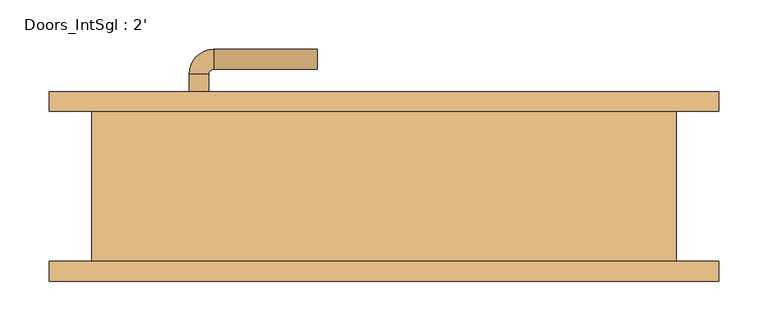
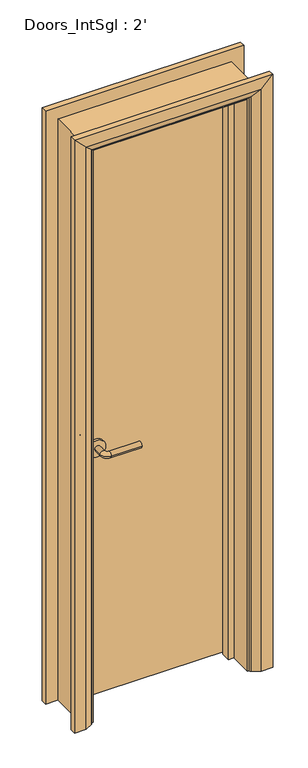
"""IFC4 building model written with IfcOpenShell, lengths in millimetres: door geometry, Doors_IntSgl : 2'."""

from ifc_helpers import new_model, si_unit, point, frame, frame_2d, origin, place, context, project, spatial, polyline, circle_curve, ellipse_curve, trimmed, segment, composite_curve, outline, extrude, faceted_brep, source, transform, mapped, element, save
from ifc_brep_helpers import plane_surface, cylinder_surface, revolved_surface, advanced_brep


def doors_intsgl_2_0e89f101(model_context):
    return source(origin(), model_context, "Body", "SolidModel", [
        advanced_brep(
        [(-197.8, 30.2, 900.0), (-177.8, 30.2, 900.0), (-177.8, 0.2, 900.0), (-197.8, 0.2, 900.0), (-172.8, -4.8, 900.0), (-172.8, -24.8, 900.0), (-67.8, -24.8, 900.0), (-67.8, -4.8, 900.0)],
        [
            (0, 1, circle_curve(frame((-187.8, 30.2, 900.0), z_axis=(0.0, 1.0, 0.0), x_axis=(1.0, 0.0, 0.0)), 10.0)),
            (1, 0, circle_curve(frame((-187.8, 30.2, 900.0), z_axis=(0.0, 1.0, 0.0), x_axis=(1.0, 0.0, 0.0)), 10.0)),
            (1, 2),
            (2, 3, circle_curve(frame((-187.8, 0.2, 900.0), z_axis=(0.0, 1.0, 0.0), x_axis=(1.0, 0.0, 0.0)), 10.0)),
            (3, 0),
            (3, 2, circle_curve(frame((-187.8, 0.2, 900.0), z_axis=(0.0, 1.0, 0.0), x_axis=(1.0, 0.0, 0.0)), 10.0)),
            (4, 5, circle_curve(frame((-172.8, -14.8, 900.0), z_axis=(-1.0, 0.0, 0.0), x_axis=(0.0, 1.0, 0.0)), 10.0)),
            (5, 3, circle_curve(frame((-172.8, 0.2, 900.0), z_axis=(0.0, 0.0, -1.0), x_axis=(-1.0, 0.0, 0.0)), 25.0)),
            (2, 4, circle_curve(frame((-172.8, 0.2, 900.0), z_axis=(0.0, 0.0, 1.0), x_axis=(-1.0, 0.0, 0.0)), 5.0)),
            (5, 4, circle_curve(frame((-172.8, -14.8, 900.0), z_axis=(-1.0, 0.0, 0.0), x_axis=(0.0, 1.0, 0.0)), 10.0)),
            (6, 7, circle_curve(frame((-67.8, -14.8, 900.0), z_axis=(1.0, 0.0, 0.0), x_axis=(0.0, 1.0, 0.0)), 10.0)),
            (7, 6, circle_curve(frame((-67.8, -14.8, 900.0), z_axis=(1.0, 0.0, 0.0), x_axis=(0.0, 1.0, 0.0)), 10.0)),
            (4, 7),
            (6, 5),
        ],
        [
            plane_surface(frame((-187.8, 30.2, 900.0), z_axis=(0.0, 1.0, 0.0), x_axis=(0.0, 0.0, 1.0))),
            cylinder_surface(frame((-187.8, 30.2, 900.0), z_axis=(0.0, 1.0, 0.0), x_axis=(1.0, 0.0, 0.0)), 10.0),
            revolved_surface(trimmed(ellipse_curve(frame((-187.8, 0.2, 900.0), z_axis=(0.0, -1.0, 0.0), x_axis=(1.0, 0.0, 0.0)), 10.0, 10.0), [point((-197.8, 0.2, 900.0))], [point((-177.8, 0.2, 900.0))], True, "CARTESIAN"), (-172.8, 0.2, 900.0), (0.0, 0.0, -1.0)),
            revolved_surface(trimmed(ellipse_curve(frame((-187.8, 0.2, 900.0), z_axis=(0.0, -1.0, 0.0), x_axis=(1.0, 0.0, 0.0)), 10.0, 10.0), [point((-177.8, 0.2, 900.0))], [point((-197.8, 0.2, 900.0))], True, "CARTESIAN"), (-172.8, 0.2, 900.0), (0.0, 0.0, -1.0)),
            plane_surface(frame((-67.8, -14.8, 900.0), z_axis=(1.0, 0.0, 0.0), x_axis=(0.0, 0.0, 1.0))),
            cylinder_surface(frame((-172.8, -14.8, 900.0), z_axis=(-1.0, 0.0, 0.0), x_axis=(0.0, 1.0, 0.0)), 10.0),
        ],
        [
            (0, [[1, 2]]),
            (1, [[3, 4, 5, -2]]),
            (1, [[-5, 6, -3, -1]]),
            (2, [[7, 8, -4, 9]]),
            (3, [[10, -9, -6, -8]]),
            (4, [[11, 12]]),
            (5, [[13, -11, 14, -7]]),
            (5, [[-14, -12, -13, -10]]),
        ],
    ),
        extrude(outline(composite_curve([segment(trimmed(circle_curve(frame_2d((900.0, -190.3)), 30.0), [point((900.0, -220.3))], [point((900.0, -160.3))], False, "CARTESIAN"), True, "CONTINUOUS"), segment(trimmed(circle_curve(frame_2d((900.0, -190.3)), 30.0), [point((900.0, -160.3))], [point((900.0, -220.3))], False, "CARTESIAN"), True, "CONTINUOUS")], self_intersect=False)), frame((0.0, 30.2, 0.0), z_axis=(0.0, 1.0, 0.0), x_axis=(0.0, 0.0, 1.0)), (0.0, 0.0, 1.0), 8.0),
        advanced_brep(
        [(-197.8, 84.2, 900.0), (-177.8, 84.2, 900.0), (-197.8, 114.2, 900.0), (-177.8, 114.2, 900.0), (-172.8, 119.2, 900.0), (-172.8, 139.2, 900.0), (-67.8, 139.2, 900.0), (-67.8, 119.2, 900.0)],
        [
            (0, 1, circle_curve(frame((-187.8, 84.2, 900.0), z_axis=(0.0, -1.0, 0.0), x_axis=(1.0, 0.0, 0.0)), 10.0)),
            (1, 0, circle_curve(frame((-187.8, 84.2, 900.0), z_axis=(0.0, -1.0, 0.0), x_axis=(1.0, 0.0, 0.0)), 10.0)),
            (0, 2),
            (2, 3, circle_curve(frame((-187.8, 114.2, 900.0), z_axis=(0.0, -1.0, 0.0), x_axis=(1.0, 0.0, 0.0)), 10.0)),
            (3, 1),
            (3, 2, circle_curve(frame((-187.8, 114.2, 900.0), z_axis=(0.0, -1.0, 0.0), x_axis=(1.0, 0.0, 0.0)), 10.0)),
            (4, 3, circle_curve(frame((-172.8, 114.2, 900.0), z_axis=(0.0, 0.0, 1.0), x_axis=(-1.0, 0.0, 0.0)), 5.0)),
            (2, 5, circle_curve(frame((-172.8, 114.2, 900.0), z_axis=(0.0, 0.0, -1.0), x_axis=(-1.0, 0.0, 0.0)), 25.0)),
            (5, 4, circle_curve(frame((-172.8, 129.2, 900.0), z_axis=(-1.0, 0.0, 0.0), x_axis=(0.0, -1.0, 0.0)), 10.0)),
            (4, 5, circle_curve(frame((-172.8, 129.2, 900.0), z_axis=(-1.0, 0.0, 0.0), x_axis=(0.0, -1.0, 0.0)), 10.0)),
            (6, 7, circle_curve(frame((-67.8, 129.2, 900.0), z_axis=(1.0, 0.0, 0.0), x_axis=(0.0, -1.0, 0.0)), 10.0)),
            (7, 6, circle_curve(frame((-67.8, 129.2, 900.0), z_axis=(1.0, 0.0, 0.0), x_axis=(0.0, -1.0, 0.0)), 10.0)),
            (5, 6),
            (7, 4),
        ],
        [
            plane_surface(frame((-187.8, 84.2, 900.0), z_axis=(0.0, -1.0, 0.0), x_axis=(0.0, 0.0, 1.0))),
            cylinder_surface(frame((-187.8, 84.2, 900.0), z_axis=(0.0, -1.0, 0.0), x_axis=(1.0, 0.0, 0.0)), 10.0),
            revolved_surface(trimmed(ellipse_curve(frame((-187.8, 114.2, 900.0), z_axis=(0.0, -1.0, 0.0), x_axis=(1.0, 0.0, 0.0)), 10.0, 10.0), [point((-197.8, 114.2, 900.0))], [point((-177.8, 114.2, 900.0))], True, "CARTESIAN"), (-172.8, 114.2, 900.0), (0.0, 0.0, -1.0)),
            revolved_surface(trimmed(ellipse_curve(frame((-187.8, 114.2, 900.0), z_axis=(0.0, -1.0, 0.0), x_axis=(1.0, 0.0, 0.0)), 10.0, 10.0), [point((-177.8, 114.2, 900.0))], [point((-197.8, 114.2, 900.0))], True, "CARTESIAN"), (-172.8, 114.2, 900.0), (0.0, 0.0, -1.0)),
            plane_surface(frame((-67.8, 129.2, 900.0), z_axis=(1.0, 0.0, 0.0), x_axis=(0.0, 0.0, 1.0))),
            cylinder_surface(frame((-172.8, 129.2, 900.0), z_axis=(-1.0, 0.0, 0.0), x_axis=(0.0, -1.0, 0.0)), 10.0),
        ],
        [
            (0, [[1, 2]]),
            (1, [[-1, 3, 4, 5]]),
            (1, [[-2, -5, 6, -3]]),
            (2, [[7, -4, 8, 9]]),
            (3, [[-8, -6, -7, 10]]),
            (4, [[11, 12]]),
            (5, [[-9, 13, -12, 14]]),
            (5, [[-10, -14, -11, -13]]),
        ],
    ),
        extrude(outline(composite_curve([segment(trimmed(circle_curve(frame_2d((900.0, -190.3)), 30.0), [point((900.0, -220.3))], [point((900.0, -160.3))], False, "CARTESIAN"), True, "CONTINUOUS"), segment(trimmed(circle_curve(frame_2d((900.0, -190.3)), 30.0), [point((900.0, -160.3))], [point((900.0, -220.3))], False, "CARTESIAN"), True, "CONTINUOUS")], self_intersect=False)), frame((0.0, 76.2, 0.0), z_axis=(0.0, 1.0, 0.0), x_axis=(0.0, 0.0, 1.0)), (0.0, 0.0, 1.0), 8.0),
        extrude(outline(polyline([(262.8, 38.2), (-262.8, 38.2), (-262.8, 76.2), (262.8, 76.2), (262.8, 38.2)])), frame((0.0, 0.0, 8.0), z_axis=(0.0, 0.0, 1.0), x_axis=(1.0, 0.0, 0.0)), (0.0, 0.0, 1.0), 2060.0),
        advanced_brep(
        [(339.8, 96.2, 0.0), (339.8, 76.2, 0.0), (269.8, 76.2, 0.0), (273.8, 82.2, 0.0), (299.8, 96.2, 0.0), (339.8, 96.2, 2145.0), (339.8, 76.2, 2145.0), (-339.8, 76.2, 2145.0), (-339.8, 76.2, 0.0), (-269.8, 76.2, 0.0), (-269.8, 76.2, 2075.0), (269.8, 76.2, 2075.0), (273.8, 82.2, 2079.0), (299.8, 96.2, 2105.0), (-299.8, 96.2, 2105.0), (-299.8, 96.2, 0.0), (-339.8, 96.2, 0.0), (-339.8, 96.2, 2145.0), (-273.8, 82.2, 0.0), (-273.8, 82.2, 2079.0)],
        [
            (0, 1),
            (1, 2),
            (2, 3, circle_curve(frame((277.8, 75.2, 0.0), z_axis=(0.0, 0.0, -1.0), x_axis=(1.0, 0.0, 0.0)), 8.0622577)),
            (3, 4),
            (4, 0),
            (0, 5),
            (5, 6),
            (6, 1),
            (6, 7),
            (7, 8),
            (8, 9),
            (9, 10),
            (10, 11),
            (11, 2),
            (11, 12, ellipse_curve(frame((277.8, 75.2, 2083.0), z_axis=(0.7071067811865475, 0.0, -0.7071067811865475), x_axis=(-0.7071067811865474, 0.0, -0.7071067811865476)), 11.4017543, 8.0622577)),
            (12, 3),
            (12, 13),
            (13, 4),
            (13, 14),
            (14, 15),
            (15, 16),
            (16, 17),
            (17, 5),
            (7, 17),
            (16, 8),
            (15, 18),
            (18, 9, circle_curve(frame((-277.8, 75.2, 0.0), z_axis=(0.0, 0.0, -1.0), x_axis=(-1.0, 0.0, 0.0)), 8.0622577)),
            (19, 10, ellipse_curve(frame((-277.8, 75.2, 2083.0), z_axis=(-0.7071067811865475, 0.0, -0.7071067811865475), x_axis=(-0.7071067811865474, 0.0, 0.7071067811865476)), 11.4017543, 8.0622577)),
            (18, 19),
            (14, 19),
            (19, 12),
        ],
        [
            plane_surface(frame((269.8, 76.2, 0.0), z_axis=(0.0, 0.0, -1.0), x_axis=(0.0, -1.0, 0.0))),
            plane_surface(frame((339.8, 96.2, 0.0), z_axis=(1.0, 0.0, 0.0), x_axis=(0.0, 0.0, 1.0))),
            plane_surface(frame((339.8, 76.2, 0.0), z_axis=(0.0, -1.0, 0.0), x_axis=(0.0, 0.0, 1.0))),
            cylinder_surface(frame((277.8, 75.2, 0.0), z_axis=(0.0, 0.0, -1.0), x_axis=(1.0, 0.0, 0.0)), 8.0622577),
            plane_surface(frame((273.8, 82.2, 0.0), z_axis=(-0.4740998230350126, 0.880471099922178, 0.0), x_axis=(0.0, 0.0, 1.0))),
            plane_surface(frame((299.8, 96.2, 0.0), z_axis=(0.0, 1.0, 0.0), x_axis=(0.0, 0.0, 1.0))),
            plane_surface(frame((-339.8, 96.2, 2145.0), z_axis=(-1.0, 0.0, 0.0), x_axis=(0.0, 0.0, -1.0))),
            plane_surface(frame((-269.8, 76.2, 0.0), z_axis=(0.0, 0.0, -1.0), x_axis=(0.0, -1.0, 0.0))),
            cylinder_surface(frame((-277.8, 75.2, 2075.0), z_axis=(0.0, 0.0, 1.0), x_axis=(-1.0, 0.0, 0.0)), 8.0622577),
            plane_surface(frame((-273.8, 82.2, 2079.0), z_axis=(0.47409982303501835, 0.8804710999221749, 0.0), x_axis=(0.0, 0.0, -1.0))),
            plane_surface(frame((339.8, 96.2, 2145.0), z_axis=(0.0, 0.0, 1.0), x_axis=(-1.0, 0.0, 0.0))),
            cylinder_surface(frame((269.8, 75.2, 2083.0), z_axis=(1.0, 0.0, 0.0), x_axis=(0.0, 0.0, 1.0)), 8.0622577),
            plane_surface(frame((273.8, 82.2, 2079.0), z_axis=(0.0, 0.8804710999221764, -0.47409982303501547), x_axis=(-1.0, 0.0, 0.0))),
        ],
        [
            (0, [[1, 2, 3, 4, 5]]),
            (1, [[-1, 6, 7, 8]]),
            (2, [[-2, -8, 9, 10, 11, 12, 13, 14]]),
            (3, [[-3, -14, 15, 16]]),
            (4, [[-4, -16, 17, 18]]),
            (5, [[-5, -18, 19, 20, 21, 22, 23, -6]]),
            (6, [[24, -22, 25, -10]]),
            (7, [[-21, 26, 27, -11, -25]]),
            (8, [[28, -12, -27, 29]]),
            (9, [[30, -29, -26, -20]]),
            (10, [[-7, -23, -24, -9]]),
            (11, [[-15, -13, -28, 31]]),
            (12, [[-17, -31, -30, -19]]),
        ],
    ),
        extrude(outline(polyline([(0.0, -264.8), (0.0, -245.8), (2051.0, -245.8), (2051.0, 245.8), (0.0, 245.8), (0.0, 264.8), (2070.0, 264.8), (2070.0, -264.8), (0.0, -264.8)])), frame((0.0, 4.2, 0.0), z_axis=(0.0, 1.0, 0.0), x_axis=(0.0, 0.0, 1.0)), (0.0, 0.0, 1.0), 32.0),
        advanced_brep(
        [(-339.8, -96.2, 0.0), (-339.8, -76.2, 0.0), (-269.8, -76.2, 0.0), (-273.8, -82.2, 0.0), (-299.8, -96.2, 0.0), (-339.8, -96.2, 2145.0), (-339.8, -76.2, 2145.0), (-269.8, -76.2, 2075.0), (-273.8, -82.2, 2079.0), (-299.8, -96.2, 2105.0), (339.8, -96.2, 0.0), (299.8, -96.2, 0.0), (273.8, -82.2, 0.0), (269.8, -76.2, 0.0), (339.8, -76.2, 0.0), (339.8, -96.2, 2145.0), (299.8, -96.2, 2105.0), (273.8, -82.2, 2079.0), (269.8, -76.2, 2075.0), (339.8, -76.2, 2145.0)],
        [
            (0, 1),
            (1, 2),
            (2, 3, circle_curve(frame((-277.8, -75.2, 0.0), z_axis=(0.0, 0.0, -1.0), x_axis=(-1.0, 0.0, 0.0)), 8.0622577)),
            (3, 4),
            (4, 0),
            (0, 5),
            (5, 6),
            (6, 1),
            (6, 7),
            (7, 2),
            (7, 8, ellipse_curve(frame((-277.8, -75.2, 2083.0), z_axis=(-0.7071067811865475, 0.0, -0.7071067811865475), x_axis=(0.7071067811865474, 0.0, -0.7071067811865476)), 11.4017543, 8.0622577)),
            (8, 3),
            (8, 9),
            (9, 4),
            (9, 5),
            (10, 11),
            (11, 12),
            (12, 13, circle_curve(frame((277.8, -75.2, 0.0), z_axis=(0.0, 0.0, -1.0), x_axis=(1.0, 0.0, 0.0)), 8.0622577)),
            (13, 14),
            (14, 10),
            (15, 16),
            (16, 11),
            (10, 15),
            (16, 17),
            (17, 12),
            (17, 18, ellipse_curve(frame((277.8, -75.2, 2083.0), z_axis=(0.7071067811865475, 0.0, -0.7071067811865475), x_axis=(0.7071067811865474, 0.0, 0.7071067811865476)), 11.4017543, 8.0622577)),
            (18, 13),
            (18, 19),
            (19, 14),
            (19, 15),
            (5, 15),
            (19, 6),
            (18, 7),
            (17, 8),
            (16, 9),
        ],
        [
            plane_surface(frame((-269.8, -149.0010989, 0.0), z_axis=(0.0, 0.0, -1.0), x_axis=(1.0, 0.0, 0.0))),
            plane_surface(frame((-339.8, -96.2, 0.0), z_axis=(-1.0, 0.0, 0.0), x_axis=(0.0, 0.0, 1.0))),
            plane_surface(frame((-339.8, -76.2, 0.0), z_axis=(0.0, 1.0, 0.0), x_axis=(0.0, 0.0, 1.0))),
            cylinder_surface(frame((-277.8, -75.2, 0.0), z_axis=(0.0, 0.0, -1.0), x_axis=(-1.0, 0.0, 0.0)), 8.0622577),
            plane_surface(frame((-273.8, -82.2, 0.0), z_axis=(0.4740998230350183, -0.8804710999221749, 0.0), x_axis=(0.0, 0.0, 1.0))),
            plane_surface(frame((-299.8, -96.2, 0.0), z_axis=(0.0, -1.0, 0.0), x_axis=(0.0, 0.0, 1.0))),
            plane_surface(frame((269.8, -149.0010989, 0.0), z_axis=(0.0, 0.0, -1.0), x_axis=(-1.0, 0.0, 0.0))),
            plane_surface(frame((299.8, -96.2, 2105.0), z_axis=(0.0, -1.0, 0.0), x_axis=(0.0, 0.0, -1.0))),
            plane_surface(frame((273.8, -82.2, 2079.0), z_axis=(-0.4740998230350183, -0.8804710999221749, 0.0), x_axis=(0.0, 0.0, -1.0))),
            cylinder_surface(frame((277.8, -75.2, 2075.0), z_axis=(0.0, 0.0, 1.0), x_axis=(1.0, 0.0, 0.0)), 8.0622577),
            plane_surface(frame((339.8, -76.2, 2145.0), z_axis=(0.0, 1.0, 0.0), x_axis=(0.0, 0.0, -1.0))),
            plane_surface(frame((339.8, -96.2, 2145.0), z_axis=(1.0, 0.0, 0.0), x_axis=(0.0, 0.0, -1.0))),
            plane_surface(frame((-339.8, -96.2, 2145.0), z_axis=(0.0, 0.0, 1.0), x_axis=(1.0, 0.0, 0.0))),
            plane_surface(frame((-339.8, -76.2, 2145.0), z_axis=(0.0, 1.0, 0.0), x_axis=(1.0, 0.0, 0.0))),
            cylinder_surface(frame((-269.8, -75.2, 2083.0), z_axis=(-1.0, 0.0, 0.0), x_axis=(0.0, 0.0, 1.0)), 8.0622577),
            plane_surface(frame((-273.8, -82.2, 2079.0), z_axis=(0.0, -0.8804710999221749, -0.4740998230350183), x_axis=(1.0, 0.0, 0.0))),
            plane_surface(frame((-299.8, -96.2, 2105.0), z_axis=(0.0, -1.0, 0.0), x_axis=(1.0, 0.0, 0.0))),
        ],
        [
            (0, [[1, 2, 3, 4, 5]]),
            (1, [[-1, 6, 7, 8]]),
            (2, [[-2, -8, 9, 10]]),
            (3, [[-3, -10, 11, 12]]),
            (4, [[-4, -12, 13, 14]]),
            (5, [[-5, -14, 15, -6]]),
            (6, [[16, 17, 18, 19, 20]]),
            (7, [[21, 22, -16, 23]]),
            (8, [[24, 25, -17, -22]]),
            (9, [[26, 27, -18, -25]]),
            (10, [[28, 29, -19, -27]]),
            (11, [[30, -23, -20, -29]]),
            (12, [[-7, 31, -30, 32]]),
            (13, [[-9, -32, -28, 33]]),
            (14, [[-11, -33, -26, 34]]),
            (15, [[-13, -34, -24, 35]]),
            (16, [[-15, -35, -21, -31]]),
        ],
    ),
        faceted_brep([(-264.8, 76.2, 0.0), (-264.8, -76.2, 0.0), (-296.8, -76.2, 0.0), (-296.8, 76.2, 0.0), (-264.8, 76.2, 2070.0), (-264.8, -76.2, 2070.0), (-296.8, -76.2, 2102.0), (-296.8, 76.2, 2102.0), (264.8, 76.2, 0.0), (296.8, 76.2, 0.0), (296.8, -76.2, 0.0), (264.8, -76.2, 0.0), (264.8, 76.2, 2070.0), (296.8, 76.2, 2102.0), (296.8, -76.2, 2102.0), (264.8, -76.2, 2070.0)], [[[0, 1, 2, 3]], [[1, 0, 4, 5]], [[2, 1, 5, 6]], [[3, 2, 6, 7]], [[0, 3, 7, 4]], [[8, 9, 10, 11]], [[12, 13, 9, 8]], [[13, 14, 10, 9]], [[14, 15, 11, 10]], [[15, 12, 8, 11]], [[5, 4, 12, 15]], [[6, 5, 15, 14]], [[7, 6, 14, 13]], [[4, 7, 13, 12]]]),
    ])


if __name__ == "__main__":
    model = new_model("IFC4")
    model_context = context("Model", 3, world=origin())
    ifc_project = project(units=[si_unit("LENGTHUNIT", "METRE", prefix="MILLI")], contexts=[model_context])
    site = spatial("IfcSite", under=ifc_project)
    building = spatial("IfcBuilding", under=site)
    placement = place(None, origin())
    doors_intsgl_2_shape = doors_intsgl_2_0e89f101(model_context)
    element("IfcDoor", 1, ObjectType="Doors_IntSgl : 2'", at=placement, inside=building, context=model_context, shape_type="MappedRepresentation", body=[
        mapped(doors_intsgl_2_shape, transform((0.0, 0.0, 0.0), x_axis=(1.0, 0.0, 0.0), y_axis=(0.0, 1.0, 0.0), z_axis=(0.0, 0.0, 1.0))),
    ])
    save(model, "model.ifc")

# Revit data of these elements
# Type "Doors_IntSgl : 2'"
#   Type Mark = "57"
#   Type Comments = "Internal Single"
#   Operation = "SingleSwingRight"
#   Manufacturer = "Revit"
#   Keynote = "L20"
#   Description = "Internal Single Door"
#   Analytic Construction = "Metal"
#   UnderCut = 8 mm
#   Tolerance = 2 mm
#   Thickness = 38 mm
#   Thermal Resistance (R) = 0.270117 (m²·K)/W
#   Structural Tolerance = 8 mm
#   StopDepth = 32 mm
#   Stop Thickness = 19 mm
#   Rough Width = 609.6 mm
#   Rough Height = 2110 mm
#   Height to Top Lock Rail = 1000 mm
#   Heat Transfer Coefficient (U) = 3.7021 W/(m²·K)
#   Handle Z Distance = 900 mm
#   Handle X Distance = 75 mm
#   Frame Thickness = 32 mm
#   Door Panel Width = 525.6 mm
#   Door Panel Thickness = 38 mm
#   Door Panel Offset = 0 mm
#   Height = 2110 mm
#   Width = 609.6 mm
#   Door Panel Height = 2060 mm
#   Architrave Setback = 5 mm
#   Vis - Ironmongery = yes
#   Material Ironmongery = Door - Handle
#   Material Frame = Door - Frame/Mullion (1)
#   Material Door = Door - Panel
#   Material Architrave = Door - Architrave
#   Visual Light Transmittance = 0
#   Solar Heat Gain Coefficient = 0
#   Function = (empty or 0)
#   Wall Closure = (empty or 0)
# Element 1 (IfcDoor, "Doors_IntSgl : 2'")
#   Materials on its faces: "Door - Architrave", "Door - Handle", "Door - Frame/Mullion (1)", "Door - Panel"
# Materials
#   "Door - Handle": colour RGB 0 0 0, transparency 0, Keynote = "P21", Cost = 0
#   "Door - Frame/Mullion (1)": class "Wood", colour RGB 212 179 113, transparency 0, Keynote = "L20", Cost = 0
#   "Door - Panel": class "Wood", colour RGB 210 159 95, transparency 0, Keynote = "L20", Cost = 0
#   "Door - Architrave": class "Wood", colour RGB 154 90 5, transparency 0, Keynote = "P20", Cost = 0
